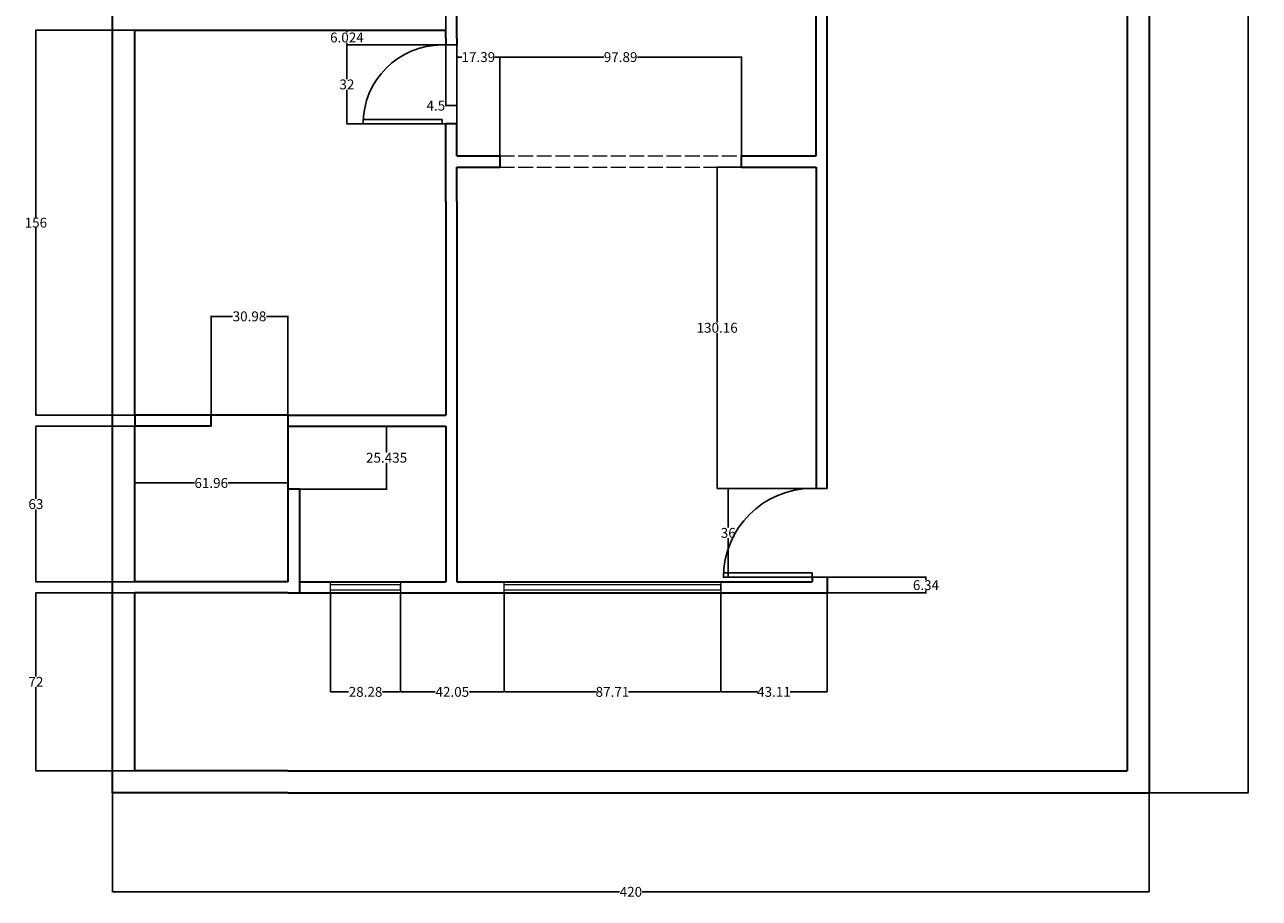
# Model space of a CAD drawing. Units: inches. Extents: x 1353 to 1853, y 16593 to 17433.
# Tile 1 of 4: x 1353 to 1853, y 16593 to 16947. Entities that reach past the tile are written whole.
import ezdxf

# ---------------------------------------------------------------- set-up
doc = ezdxf.new("R2010")
doc.units = ezdxf.units.IN
doc.header["$MEASUREMENT"] = 0
doc.linetypes.add('ACAD_ISO02W100', pattern=[15, 12, -3])
for name, color, linetype, lineweight in [('A-ANNO-DIMS', 2, 'Continuous', 18), ('A-DOOR', 3, 'Continuous', 25), ('A-GLAZ', 4, 'Continuous', 18), ('A-WALL', 7, 'Continuous', 35)]:
    doc.layers.add(name, color=color, linetype=linetype, lineweight=lineweight)
doc.layers.add('A-WALL-OVHD', color=51, linetype='ACAD_ISO02W100', lineweight=18, true_color=0xf8f6b0)
doc.styles.get("Standard").update_dxf_attribs({"font": 'arial.ttf'})
doc.dimstyles.get("Standard").update_dxf_attribs({"dimtxt": 4, "dimasz": 0.18, "dimexe": 0.18, "dimexo": 0.0625, "dimgap": 0.09, "dimtad": 0, "dimtih": 1, "dimtoh": 1, "dimdec": 0, "dimzin": 0, "dimdsep": 46, "dimlunit": 3, "dimtxsty": 'Standard', "dimcen": 0.09, "dimadec": 0, "dimazin": 0, "dimtfac": 1, "dimtdec": 0, "dimtofl": 0, "dimtmove": 0, "dimatfit": 3, "dimfxl": 1, "dimtolj": 1, "dimtzin": 0, "dimarcsym": 0})

# ---------------------------------------------------------------- blocks, each defined once
blk = doc.blocks.new('*U4')
for p, q in [((0, 0), (0, -6)), ((32, 0), (32, -6))]:
    blk.add_line(p, q)
blk.add_lwpolyline([(0, 0), (0, 32), (1.75, 32), (1.75, 0)], close=True)
blk.add_arc((0, 0), 32, 0, 90)
blk = doc.blocks.new('*U3')
for p, q in [((0, 0), (0, -6)), ((36, 0), (36, -6))]:
    blk.add_line(p, q)
blk.add_lwpolyline([(0, 0), (0, 36), (1.75, 36), (1.75, 0)], close=True)
blk.add_arc((0, 0), 36, 0, 90)
blk = doc.blocks.new('*D13')
at = {"layer": 'A-ANNO-DIMS', "color": 0, "lineweight": -2, "transparency": 16777216}
for p, q in [((1388.88, 16635.72), (1388.88, 16595.55)), ((1808.88, 16635.72), (1808.88, 16595.55)), ((1389.06, 16595.73), (1594.3, 16595.73)), ((1808.7, 16595.73), (1603.47, 16595.73))]:
    blk.add_line(p, q, dxfattribs=at)
at = {"layer": 'A-ANNO-DIMS', "color": 0, "transparency": 16777216}
for points in [[(1389.06, 16595.76), (1389.06, 16595.7), (1388.88, 16595.73)], [(1808.7, 16595.76), (1808.7, 16595.7), (1808.88, 16595.73)]]:
    blk.add_solid(points, dxfattribs=at)
at = {"layer": 'Defpoints', "color": 0, "transparency": 16777216}
for p in [(1388.88, 16635.78), (1808.88, 16635.78), (1808.88, 16595.73)]:
    blk.add_point(p, dxfattribs=at)
at = {"layer": 'A-ANNO-DIMS', "color": 0, "transparency": 16777216, "insert": (1598.88, 16595.73), "char_height": 4, "attachment_point": 5}
blk.add_mtext('\\A1;420', dxfattribs=at)
blk = doc.blocks.new('*D14')
at = {"layer": 'A-ANNO-DIMS', "color": 0, "lineweight": -2, "transparency": 16777216}
for p, q in [((1808.95, 17432.78), (1849.11, 17432.78)), ((1848.93, 17432.6), (1848.93, 17036.41)), ((1848.93, 16635.96), (1848.93, 17032.15)), ((1808.95, 16635.78), (1849.11, 16635.78))]:
    blk.add_line(p, q, dxfattribs=at)
at = {"layer": 'A-ANNO-DIMS', "color": 0, "transparency": 16777216}
for points in [[(1848.9, 17432.6), (1848.96, 17432.6), (1848.93, 17432.78)], [(1848.9, 16635.96), (1848.96, 16635.96), (1848.93, 16635.78)]]:
    blk.add_solid(points, dxfattribs=at)
at = {"layer": 'Defpoints', "color": 0, "transparency": 16777216}
for p in [(1808.88, 17432.78), (1848.93, 17432.78), (1808.88, 16635.78)]:
    blk.add_point(p, dxfattribs=at)
at = {"layer": 'A-ANNO-DIMS', "color": 0, "transparency": 16777216, "insert": (1848.93, 17034.28), "char_height": 4, "attachment_point": 5}
blk.add_mtext('\\A1;797', dxfattribs=at)
blk = doc.blocks.new('*D20')
at = {"layer": 'A-ANNO-DIMS', "color": 0, "lineweight": -2, "transparency": 16777216}
for p, q in [((1397.82, 16944.78), (1357.65, 16944.78)), ((1357.83, 16944.6), (1357.83, 16868.91)), ((1357.83, 16788.96), (1357.83, 16864.65)), ((1397.82, 16788.78), (1357.65, 16788.78))]:
    blk.add_line(p, q, dxfattribs=at)
at = {"layer": 'A-ANNO-DIMS', "color": 0, "transparency": 16777216}
for points in [[(1357.8, 16944.6), (1357.86, 16944.6), (1357.83, 16944.78)], [(1357.8, 16788.96), (1357.86, 16788.96), (1357.83, 16788.78)]]:
    blk.add_solid(points, dxfattribs=at)
at = {"layer": 'Defpoints', "color": 0, "transparency": 16777216}
for p in [(1357.83, 16944.78), (1397.88, 16944.78), (1397.88, 16788.78)]:
    blk.add_point(p, dxfattribs=at)
at = {"layer": 'A-ANNO-DIMS', "color": 0, "transparency": 16777216, "insert": (1357.83, 16866.78), "char_height": 4, "attachment_point": 5}
blk.add_mtext('\\A1;156', dxfattribs=at)
blk = doc.blocks.new('*D21')
at = {"layer": 'A-ANNO-DIMS', "color": 0, "lineweight": -2, "transparency": 16777216}
for p, q in [((1397.82, 16784.28), (1357.65, 16784.28)), ((1357.83, 16784.1), (1357.83, 16754.91)), ((1357.83, 16721.46), (1357.83, 16750.65)), ((1397.82, 16721.28), (1357.65, 16721.28))]:
    blk.add_line(p, q, dxfattribs=at)
at = {"layer": 'A-ANNO-DIMS', "color": 0, "transparency": 16777216}
for points in [[(1357.8, 16784.1), (1357.86, 16784.1), (1357.83, 16784.28)], [(1357.8, 16721.46), (1357.86, 16721.46), (1357.83, 16721.28)]]:
    blk.add_solid(points, dxfattribs=at)
at = {"layer": 'Defpoints', "color": 0, "transparency": 16777216}
for p in [(1357.83, 16784.28), (1397.88, 16784.28), (1397.88, 16721.28)]:
    blk.add_point(p, dxfattribs=at)
at = {"layer": 'A-ANNO-DIMS', "color": 0, "transparency": 16777216, "insert": (1357.83, 16752.78), "char_height": 4, "attachment_point": 5}
blk.add_mtext('\\A1;63', dxfattribs=at)
blk = doc.blocks.new('*D22')
at = {"layer": 'A-ANNO-DIMS', "color": 0, "lineweight": -2, "transparency": 16777216}
for p, q in [((1397.82, 16716.78), (1357.65, 16716.78)), ((1357.83, 16716.6), (1357.83, 16682.88)), ((1357.83, 16644.96), (1357.83, 16678.68)), ((1397.82, 16644.78), (1357.65, 16644.78))]:
    blk.add_line(p, q, dxfattribs=at)
at = {"layer": 'A-ANNO-DIMS', "color": 0, "transparency": 16777216}
for points in [[(1357.8, 16716.6), (1357.86, 16716.6), (1357.83, 16716.78)], [(1357.8, 16644.96), (1357.86, 16644.96), (1357.83, 16644.78)]]:
    blk.add_solid(points, dxfattribs=at)
at = {"layer": 'Defpoints', "color": 0, "transparency": 16777216}
for p in [(1357.83, 16716.78), (1397.88, 16716.78), (1397.88, 16644.78)]:
    blk.add_point(p, dxfattribs=at)
at = {"layer": 'A-ANNO-DIMS', "color": 0, "transparency": 16777216, "insert": (1357.83, 16680.78), "char_height": 4, "attachment_point": 5}
blk.add_mtext('\\A1;72', dxfattribs=at)
blk = doc.blocks.new('*D29')
at = {"layer": 'A-ANNO-DIMS', "color": 0, "lineweight": -2, "transparency": 16777216}
for p, q in [((1673.82, 16889.28), (1633.65, 16889.28)), ((1633.83, 16889.1), (1633.83, 16826.33)), ((1633.83, 16759.3), (1633.83, 16822.07)), ((1673.82, 16759.12), (1633.65, 16759.12))]:
    blk.add_line(p, q, dxfattribs=at)
at = {"layer": 'A-ANNO-DIMS', "color": 0, "transparency": 16777216}
for points in [[(1633.8, 16889.1), (1633.86, 16889.1), (1633.83, 16889.28)], [(1633.8, 16759.3), (1633.86, 16759.3), (1633.83, 16759.12)]]:
    blk.add_solid(points, dxfattribs=at)
at = {"layer": 'Defpoints', "color": 0, "transparency": 16777216}
for p in [(1633.83, 16889.28), (1673.88, 16889.28), (1673.88, 16759.12)]:
    blk.add_point(p, dxfattribs=at)
at = {"layer": 'A-ANNO-DIMS', "color": 0, "transparency": 16777216, "insert": (1633.83, 16824.2), "char_height": 4, "attachment_point": 5}
blk.add_mtext('\\A1;130.16', dxfattribs=at)
blk = doc.blocks.new('*D32')
at = {"layer": 'A-ANNO-DIMS', "color": 0, "lineweight": -2, "transparency": 16777216}
for p, q in [((1397.88, 16721.34), (1397.88, 16761.51)), ((1398.06, 16761.33), (1422.02, 16761.33)), ((1459.67, 16761.33), (1435.71, 16761.33)), ((1459.85, 16721.34), (1459.85, 16761.51))]:
    blk.add_line(p, q, dxfattribs=at)
at = {"layer": 'A-ANNO-DIMS', "color": 0, "transparency": 16777216}
for points in [[(1398.06, 16761.36), (1398.06, 16761.3), (1397.88, 16761.33)], [(1459.67, 16761.36), (1459.67, 16761.3), (1459.85, 16761.33)]]:
    blk.add_solid(points, dxfattribs=at)
at = {"layer": 'Defpoints', "color": 0, "transparency": 16777216}
for p in [(1459.85, 16761.33), (1397.88, 16721.28), (1459.85, 16721.28)]:
    blk.add_point(p, dxfattribs=at)
at = {"layer": 'A-ANNO-DIMS', "color": 0, "transparency": 16777216, "insert": (1428.87, 16761.33), "char_height": 4, "attachment_point": 5}
blk.add_mtext('\\A1;61.96', dxfattribs=at)
blk = doc.blocks.new('*D33')
at = {"layer": 'A-ANNO-DIMS', "color": 0, "lineweight": -2, "transparency": 16777216}
for p, q in [((1523.88, 16954.18), (1523.88, 16914.01)), ((1528.38, 16954.18), (1528.38, 16914.01)), ((1523.88, 16914.19), (1523.7, 16914.19)), ((1528.2, 16914.19), (1524.06, 16914.19))]:
    blk.add_line(p, q, dxfattribs=at)
at = {"layer": 'A-ANNO-DIMS', "color": 0, "transparency": 16777216}
for points in [[(1524.06, 16914.22), (1524.06, 16914.16), (1523.88, 16914.19)], [(1528.2, 16914.22), (1528.2, 16914.16), (1528.38, 16914.19)]]:
    blk.add_solid(points, dxfattribs=at)
at = {"layer": 'Defpoints', "color": 0, "transparency": 16777216}
for p in [(1523.88, 16954.24), (1528.38, 16954.24), (1523.88, 16914.19)]:
    blk.add_point(p, dxfattribs=at)
at = {"layer": 'A-ANNO-DIMS', "color": 0, "transparency": 16777216, "insert": (1519.88, 16914.19), "char_height": 4, "attachment_point": 5}
blk.add_mtext('\\A1;4.5', dxfattribs=at)
blk = doc.blocks.new('*D47')
at = {"layer": 'A-ANNO-DIMS', "color": 0, "lineweight": -2, "transparency": 16777216}
for p, q in [((1477.24, 16716.72), (1477.24, 16676.55)), ((1505.52, 16716.72), (1505.52, 16676.55)), ((1477.42, 16676.73), (1484.5, 16676.73)), ((1505.34, 16676.73), (1498.26, 16676.73))]:
    blk.add_line(p, q, dxfattribs=at)
at = {"layer": 'A-ANNO-DIMS', "color": 0, "transparency": 16777216}
for points in [[(1477.42, 16676.76), (1477.42, 16676.7), (1477.24, 16676.73)], [(1505.34, 16676.76), (1505.34, 16676.7), (1505.52, 16676.73)]]:
    blk.add_solid(points, dxfattribs=at)
at = {"layer": 'Defpoints', "color": 0, "transparency": 16777216}
for p in [(1477.24, 16716.78), (1505.52, 16716.78), (1477.24, 16676.73)]:
    blk.add_point(p, dxfattribs=at)
at = {"layer": 'A-ANNO-DIMS', "color": 0, "transparency": 16777216, "insert": (1491.38, 16676.73), "char_height": 4, "attachment_point": 5}
blk.add_mtext('\\A1;28.28', dxfattribs=at)
blk = doc.blocks.new('*D48')
at = {"layer": 'A-ANNO-DIMS', "color": 0, "lineweight": -2, "transparency": 16777216}
for p, q in [((1547.57, 16716.72), (1547.57, 16676.55)), ((1635.28, 16716.72), (1635.28, 16676.55)), ((1547.75, 16676.73), (1584.96, 16676.73)), ((1635.1, 16676.73), (1597.88, 16676.73))]:
    blk.add_line(p, q, dxfattribs=at)
at = {"layer": 'A-ANNO-DIMS', "color": 0, "transparency": 16777216}
for points in [[(1547.75, 16676.76), (1547.75, 16676.7), (1547.57, 16676.73)], [(1635.1, 16676.76), (1635.1, 16676.7), (1635.28, 16676.73)]]:
    blk.add_solid(points, dxfattribs=at)
at = {"layer": 'Defpoints', "color": 0, "transparency": 16777216}
for p in [(1547.57, 16716.78), (1635.28, 16716.78), (1547.57, 16676.73)]:
    blk.add_point(p, dxfattribs=at)
at = {"layer": 'A-ANNO-DIMS', "color": 0, "transparency": 16777216, "insert": (1591.42, 16676.73), "char_height": 4, "attachment_point": 5}
blk.add_mtext('\\A1;87.71', dxfattribs=at)
blk = doc.blocks.new('*D49')
at = {"layer": 'A-ANNO-DIMS', "color": 0, "lineweight": -2, "transparency": 16777216}
for p, q in [((1505.52, 16716.72), (1505.52, 16676.55)), ((1547.57, 16716.72), (1547.57, 16676.55)), ((1505.7, 16676.73), (1519.61, 16676.73)), ((1547.39, 16676.73), (1533.48, 16676.73))]:
    blk.add_line(p, q, dxfattribs=at)
at = {"layer": 'A-ANNO-DIMS', "color": 0, "transparency": 16777216}
for points in [[(1505.7, 16676.76), (1505.7, 16676.7), (1505.52, 16676.73)], [(1547.39, 16676.76), (1547.39, 16676.7), (1547.57, 16676.73)]]:
    blk.add_solid(points, dxfattribs=at)
at = {"layer": 'Defpoints', "color": 0, "transparency": 16777216}
for p in [(1505.52, 16716.78), (1547.57, 16716.78), (1505.52, 16676.73)]:
    blk.add_point(p, dxfattribs=at)
at = {"layer": 'A-ANNO-DIMS', "color": 0, "transparency": 16777216, "insert": (1526.54, 16676.73), "char_height": 4, "attachment_point": 5}
blk.add_mtext('\\A1;42.05', dxfattribs=at)
blk = doc.blocks.new('*D50')
at = {"layer": 'A-ANNO-DIMS', "color": 0, "lineweight": -2, "transparency": 16777216}
for p, q in [((1635.28, 16716.72), (1635.28, 16676.55)), ((1678.38, 16716.72), (1678.38, 16676.55)), ((1635.46, 16676.73), (1650.3, 16676.73)), ((1678.2, 16676.73), (1663.36, 16676.73))]:
    blk.add_line(p, q, dxfattribs=at)
at = {"layer": 'A-ANNO-DIMS', "color": 0, "transparency": 16777216}
for points in [[(1635.46, 16676.76), (1635.46, 16676.7), (1635.28, 16676.73)], [(1678.2, 16676.76), (1678.2, 16676.7), (1678.38, 16676.73)]]:
    blk.add_solid(points, dxfattribs=at)
at = {"layer": 'Defpoints', "color": 0, "transparency": 16777216}
for p in [(1635.28, 16716.78), (1678.38, 16716.78), (1635.28, 16676.73)]:
    blk.add_point(p, dxfattribs=at)
at = {"layer": 'A-ANNO-DIMS', "color": 0, "transparency": 16777216, "insert": (1656.83, 16676.73), "char_height": 4, "attachment_point": 5}
blk.add_mtext('\\A1;43.11', dxfattribs=at)
blk = doc.blocks.new('*D60')
at = {"layer": 'A-ANNO-DIMS', "color": 0, "lineweight": -2, "transparency": 16777216}
for p, q in [((1523.82, 16938.76), (1483.65, 16938.76)), ((1483.83, 16938.58), (1483.83, 16924.89)), ((1483.83, 16906.94), (1483.83, 16920.62)), ((1523.82, 16906.76), (1483.65, 16906.76))]:
    blk.add_line(p, q, dxfattribs=at)
at = {"layer": 'A-ANNO-DIMS', "color": 0, "transparency": 16777216}
for points in [[(1483.8, 16938.58), (1483.86, 16938.58), (1483.83, 16938.76)], [(1483.8, 16906.94), (1483.86, 16906.94), (1483.83, 16906.76)]]:
    blk.add_solid(points, dxfattribs=at)
at = {"layer": 'Defpoints', "color": 0, "transparency": 16777216}
for p in [(1483.83, 16938.76), (1523.88, 16938.76), (1523.88, 16906.76)]:
    blk.add_point(p, dxfattribs=at)
at = {"layer": 'A-ANNO-DIMS', "color": 0, "transparency": 16777216, "insert": (1483.83, 16922.76), "char_height": 4, "attachment_point": 5}
blk.add_mtext('\\A1;32', dxfattribs=at)
blk = doc.blocks.new('*D63')
at = {"layer": 'A-ANNO-DIMS', "color": 0, "lineweight": -2, "transparency": 16777216}
for p, q in [((1678.32, 16759.12), (1638.15, 16759.12)), ((1638.33, 16758.94), (1638.33, 16743.25)), ((1638.33, 16723.3), (1638.33, 16738.99)), ((1678.32, 16723.12), (1638.15, 16723.12))]:
    blk.add_line(p, q, dxfattribs=at)
at = {"layer": 'A-ANNO-DIMS', "color": 0, "transparency": 16777216}
for points in [[(1638.3, 16758.94), (1638.36, 16758.94), (1638.33, 16759.12)], [(1638.3, 16723.3), (1638.36, 16723.3), (1638.33, 16723.12)]]:
    blk.add_solid(points, dxfattribs=at)
at = {"layer": 'Defpoints', "color": 0, "transparency": 16777216}
for p in [(1638.33, 16759.12), (1678.38, 16759.12), (1678.38, 16723.12)]:
    blk.add_point(p, dxfattribs=at)
at = {"layer": 'A-ANNO-DIMS', "color": 0, "transparency": 16777216, "insert": (1638.33, 16741.12), "char_height": 4, "attachment_point": 5}
blk.add_mtext('\\A1;36', dxfattribs=at)
blk = doc.blocks.new('*D64')
at = {"layer": 'A-ANNO-DIMS', "color": 0, "lineweight": -2, "transparency": 16777216}
for p, q in [((1545.78, 16893.84), (1545.78, 16934.01)), ((1545.96, 16933.83), (1587.88, 16933.83)), ((1643.48, 16933.83), (1601.56, 16933.83)), ((1643.66, 16893.84), (1643.66, 16934.01))]:
    blk.add_line(p, q, dxfattribs=at)
at = {"layer": 'A-ANNO-DIMS', "color": 0, "transparency": 16777216}
for points in [[(1545.96, 16933.86), (1545.96, 16933.8), (1545.78, 16933.83)], [(1643.48, 16933.86), (1643.48, 16933.8), (1643.66, 16933.83)]]:
    blk.add_solid(points, dxfattribs=at)
at = {"layer": 'Defpoints', "color": 0, "transparency": 16777216}
for p in [(1643.66, 16933.83), (1545.78, 16893.78), (1643.66, 16893.78)]:
    blk.add_point(p, dxfattribs=at)
at = {"layer": 'A-ANNO-DIMS', "color": 0, "transparency": 16777216, "insert": (1594.72, 16933.83), "char_height": 4, "attachment_point": 5}
blk.add_mtext('\\A1;97.89', dxfattribs=at)
blk = doc.blocks.new('*D65')
at = {"layer": 'A-ANNO-DIMS', "color": 0, "lineweight": -2, "transparency": 16777216}
for p, q in [((1528.38, 16893.84), (1528.38, 16934.01)), ((1528.56, 16933.83), (1530.43, 16933.83)), ((1545.6, 16933.83), (1543.73, 16933.83)), ((1545.78, 16893.84), (1545.78, 16934.01))]:
    blk.add_line(p, q, dxfattribs=at)
at = {"layer": 'A-ANNO-DIMS', "color": 0, "transparency": 16777216}
for points in [[(1528.56, 16933.86), (1528.56, 16933.8), (1528.38, 16933.83)], [(1545.6, 16933.86), (1545.6, 16933.8), (1545.78, 16933.83)]]:
    blk.add_solid(points, dxfattribs=at)
at = {"layer": 'Defpoints', "color": 0, "transparency": 16777216}
for p in [(1545.78, 16933.83), (1528.38, 16893.78), (1545.78, 16893.78)]:
    blk.add_point(p, dxfattribs=at)
at = {"layer": 'A-ANNO-DIMS', "color": 0, "transparency": 16777216, "insert": (1537.08, 16933.83), "char_height": 4, "attachment_point": 5}
blk.add_mtext('\\A1;17.39', dxfattribs=at)
blk = doc.blocks.new('*D66')
at = {"layer": 'A-ANNO-DIMS', "color": 0, "lineweight": -2, "transparency": 16777216}
for p, q in [((1428.87, 16788.84), (1428.87, 16829.01)), ((1429.05, 16828.83), (1437.51, 16828.83)), ((1459.67, 16828.83), (1451.2, 16828.83)), ((1459.85, 16788.84), (1459.85, 16829.01))]:
    blk.add_line(p, q, dxfattribs=at)
at = {"layer": 'A-ANNO-DIMS', "color": 0, "transparency": 16777216}
for points in [[(1429.05, 16828.86), (1429.05, 16828.8), (1428.87, 16828.83)], [(1459.67, 16828.86), (1459.67, 16828.8), (1459.85, 16828.83)]]:
    blk.add_solid(points, dxfattribs=at)
at = {"layer": 'Defpoints', "color": 0, "transparency": 16777216}
for p in [(1459.85, 16828.83), (1428.87, 16788.78), (1459.85, 16788.78)]:
    blk.add_point(p, dxfattribs=at)
at = {"layer": 'A-ANNO-DIMS', "color": 0, "transparency": 16777216, "insert": (1444.36, 16828.83), "char_height": 4, "attachment_point": 5}
blk.add_mtext('\\A1;30.98', dxfattribs=at)
blk = doc.blocks.new('*D67')
at = {"layer": 'A-ANNO-DIMS', "color": 0, "lineweight": -2, "transparency": 16777216}
for p, q in [((1459.91, 16784.28), (1500.08, 16784.28)), ((1499.9, 16784.1), (1499.9, 16773.7)), ((1499.9, 16759.03), (1499.9, 16769.43)), ((1459.91, 16758.85), (1500.08, 16758.85))]:
    blk.add_line(p, q, dxfattribs=at)
at = {"layer": 'A-ANNO-DIMS', "color": 0, "transparency": 16777216}
for points in [[(1499.87, 16784.1), (1499.93, 16784.1), (1499.9, 16784.28)], [(1499.87, 16759.03), (1499.93, 16759.03), (1499.9, 16758.85)]]:
    blk.add_solid(points, dxfattribs=at)
at = {"layer": 'Defpoints', "color": 0, "transparency": 16777216}
for p in [(1459.85, 16784.28), (1459.85, 16758.85), (1499.9, 16758.85)]:
    blk.add_point(p, dxfattribs=at)
at = {"layer": 'A-ANNO-DIMS', "color": 0, "transparency": 16777216, "insert": (1499.9, 16771.56), "char_height": 4, "attachment_point": 5}
blk.add_mtext('\\A1;25.435', dxfattribs=at)
blk = doc.blocks.new('*D77')
at = {"layer": 'A-ANNO-DIMS', "color": 0, "lineweight": -2, "transparency": 16777216}
for p, q in [((1523.82, 16944.78), (1483.65, 16944.78)), ((1483.83, 16944.6), (1483.83, 16943.9)), ((1523.82, 16938.76), (1483.65, 16938.76)), ((1483.83, 16938.94), (1483.83, 16939.64))]:
    blk.add_line(p, q, dxfattribs=at)
at = {"layer": 'A-ANNO-DIMS', "color": 0, "transparency": 16777216}
for points in [[(1483.8, 16944.6), (1483.86, 16944.6), (1483.83, 16944.78)], [(1483.8, 16938.94), (1483.86, 16938.94), (1483.83, 16938.76)]]:
    blk.add_solid(points, dxfattribs=at)
at = {"layer": 'Defpoints', "color": 0, "transparency": 16777216}
for p in [(1483.83, 16944.78), (1523.88, 16944.78), (1523.88, 16938.76)]:
    blk.add_point(p, dxfattribs=at)
at = {"layer": 'A-ANNO-DIMS', "color": 0, "transparency": 16777216, "insert": (1483.83, 16941.77), "char_height": 4, "attachment_point": 5}
blk.add_mtext('\\A1;6.024', dxfattribs=at)
blk = doc.blocks.new('*D79')
at = {"layer": 'A-ANNO-DIMS', "color": 0, "lineweight": -2, "transparency": 16777216}
for p, q in [((1678.45, 16723.12), (1718.61, 16723.12)), ((1718.43, 16722.94), (1718.43, 16722.08)), ((1678.45, 16716.78), (1718.61, 16716.78)), ((1718.43, 16716.96), (1718.43, 16717.82))]:
    blk.add_line(p, q, dxfattribs=at)
at = {"layer": 'A-ANNO-DIMS', "color": 0, "transparency": 16777216}
for points in [[(1718.4, 16722.94), (1718.46, 16722.94), (1718.43, 16723.12)], [(1718.4, 16716.96), (1718.46, 16716.96), (1718.43, 16716.78)]]:
    blk.add_solid(points, dxfattribs=at)
at = {"layer": 'Defpoints', "color": 0, "transparency": 16777216}
for p in [(1678.38, 16723.12), (1678.38, 16716.78), (1718.43, 16716.78)]:
    blk.add_point(p, dxfattribs=at)
at = {"layer": 'A-ANNO-DIMS', "color": 0, "transparency": 16777216, "insert": (1718.43, 16719.95), "char_height": 4, "attachment_point": 5}
blk.add_mtext('\\A1;6.34', dxfattribs=at)

msp = doc.modelspace()

# ---------------------------------------------------------------- linework, layer by layer
at = {"layer": 'A-GLAZ'}
for p, q in [((1477.2369, 16716.7809), (1477.2369, 16721.2809)), ((1477.2369, 16721.2809), (1505.5194, 16721.2809)), ((1505.5194, 16721.2809), (1505.5194, 16716.7809)), ((1547.5656, 16716.7809), (1547.5656, 16721.2809)), ((1547.5656, 16721.2809), (1635.2751, 16721.2809)), ((1635.2751, 16721.2809), (1635.2751, 16721.2809)), ((1635.2751, 16721.2809), (1635.2751, 16716.7809)), ((1505.5194, 16720.0396), (1477.2369, 16720.0396)), ((1477.2369, 16720.0396), (1477.2369, 16720.0396)), ((1477.2369, 16716.7809), (1477.2369, 16718.023)), ((1477.2369, 16718.023), (1505.5194, 16718.023)), ((1505.5194, 16716.7809), (1477.2369, 16716.7809)), ((1505.5194, 16718.023), (1505.5194, 16720.0396)), ((1635.2751, 16720.0306), (1547.5656, 16720.0306)), ((1547.5656, 16716.7809), (1547.5656, 16718.014)), ((1547.5656, 16718.014), (1635.2751, 16718.014)), ((1635.2751, 16716.7809), (1547.5656, 16716.7809)), ((1635.2751, 16718.014), (1635.2751, 16720.0306))]:
    msp.add_line(p, q, dxfattribs=at)
at = {"layer": 'A-WALL'}
for p, q in [((1388.8844, 16635.7809), (1388.8844, 17432.7809)), ((1808.8844, 17432.7809), (1808.8844, 16635.7809)), ((1799.8844, 17087.7809), (1799.8844, 16644.7809)), ((1673.8844, 16893.7809), (1673.8844, 17047.277)), ((1678.3844, 16759.1207), (1678.3844, 17047.277)), ((1528.3844, 16944.7809), (1528.3844, 16954.2398)), ((1397.8844, 16944.7809), (1459.8459, 16944.7809)), ((1397.8844, 16875.2834), (1397.8844, 16944.7809)), ((1459.8459, 16944.7809), (1523.8844, 16944.7809)), ((1523.8844, 16941.5554), (1523.8844, 16944.7809)), ((1523.8844, 16941.5554), (1523.8844, 16938.7569)), ((1528.3844, 16941.5554), (1528.3844, 16944.7809)), ((1528.3844, 16941.5554), (1528.3844, 16938.7569)), ((1523.8844, 16875.2834), (1523.8844, 16906.7569)), ((1528.3844, 16906.7569), (1523.8844, 16906.7569)), ((1528.3844, 16893.7809), (1528.3844, 16906.7569)), ((1528.3844, 16893.7809), (1545.7758, 16893.7809)), ((1545.7758, 16893.7809), (1545.7758, 16889.2809)), ((1643.664, 16889.2809), (1643.664, 16893.7809)), ((1643.664, 16893.7809), (1673.8844, 16893.7809)), ((1528.3844, 16875.2834), (1528.3844, 16889.2809)), ((1528.3844, 16889.2809), (1545.7758, 16889.2809)), ((1643.664, 16889.2809), (1673.8844, 16889.2809)), ((1673.8844, 16889.2809), (1673.8844, 16763.1207)), ((1397.8844, 16788.7809), (1397.8844, 16877.2809)), ((1523.8844, 16875.2834), (1523.8844, 16788.7809)), ((1528.3844, 16875.2834), (1528.3844, 16784.2809)), ((1459.8459, 16788.7809), (1397.8844, 16788.7809)), ((1428.8651, 16788.7809), (1397.8844, 16788.7809)), ((1397.8844, 16788.7809), (1397.8844, 16784.2809)), ((1428.8651, 16784.2809), (1428.8651, 16788.7809)), ((1459.8459, 16788.7809), (1523.8844, 16788.7809)), ((1459.8459, 16788.7809), (1459.8459, 16721.2809)), ((1428.8651, 16784.2809), (1397.8844, 16784.2809)), ((1397.8844, 16721.2809), (1397.8844, 16784.2809)), ((1459.8459, 16784.2809), (1523.8844, 16784.2809)), ((1523.8844, 16784.2809), (1523.8844, 16721.2809)), ((1528.3844, 16784.2809), (1528.3844, 16721.2809)), ((1673.8844, 16763.1207), (1673.8844, 16759.1207)), ((1464.8177, 16758.8459), (1459.8459, 16758.8459)), ((1464.8177, 16716.7809), (1464.8177, 16758.8459)), ((1459.8459, 16721.2809), (1397.8844, 16721.2809)), ((1464.8177, 16721.2809), (1523.8844, 16721.2809)), ((1528.3844, 16721.2809), (1672.3844, 16721.2809)), ((1672.3844, 16721.2809), (1672.1111, 16721.2809)), ((1672.3844, 16723.1207), (1672.3844, 16721.2809)), ((1678.3844, 16723.1207), (1678.3844, 16716.7809)), ((1397.8844, 16644.7809), (1397.8844, 16716.7809)), ((1459.8459, 16716.7809), (1397.8844, 16716.7809)), ((1459.8459, 16716.7809), (1678.3844, 16716.7809)), ((1459.8459, 16716.7809), (1464.8177, 16716.7809)), ((1459.8459, 16644.7809), (1397.8844, 16644.7809)), ((1459.8459, 16644.7809), (1528.3844, 16644.7809)), ((1528.3844, 16644.7809), (1678.3844, 16644.7809)), ((1678.3844, 16644.7809), (1799.8844, 16644.7809)), ((1397.8844, 16635.7809), (1388.8844, 16635.7809)), ((1459.8459, 16635.7809), (1397.8844, 16635.7809)), ((1459.8459, 16635.7809), (1528.3844, 16635.7809)), ((1528.3844, 16635.7809), (1808.8844, 16635.7809))]:
    msp.add_line(p, q, dxfattribs=at)
at = {"layer": 'A-WALL-OVHD', "ltscale": 0.5}
for p, q in [((1545.7758, 16893.7809), (1643.664, 16893.7809)), ((1545.7758, 16889.2809), (1643.664, 16889.2809))]:
    msp.add_line(p, q, dxfattribs=at)

# ---------------------------------------------------------------- block references
at = {"layer": 'A-DOOR', "rotation": 90}
for name, p in [('*U4', (1522.3844, 16906.7569)), ('*U3', (1672.3844, 16723.1207))]:
    msp.add_blockref(name, p, dxfattribs=at)

# ---------------------------------------------------------------- dimensions: what is measured, and where the dimension line sits
at = {"layer": 'A-ANNO-DIMS'}
for base, p1, p2, angle, override, picture, middle in [((1848.9344, 17432.7809), (1808.8844, 16635.7809), (1808.8844, 17432.7809), 90, {"dimdec": 0, "dimlfac": 1, "dimrnd": 0, "dimzin": 0, "dimdsep": 46, "dimlunit": 2}, '*D14', (1848.9344, 17034.2809)), ((1523.8844, 16914.1898), (1528.3844, 16954.2398), (1523.8844, 16954.2398), 180, {"dimdec": 1, "dimlfac": 1, "dimrnd": 0, "dimzin": 0, "dimdsep": 46, "dimlunit": 2}, '*D33', (1519.8777, 16914.1898)), ((1357.8344, 16944.7809), (1397.8844, 16788.7809), (1397.8844, 16944.7809), 90, {"dimdec": 0, "dimlfac": 1, "dimrnd": 0, "dimzin": 0, "dimdsep": 46, "dimlunit": 2}, '*D20', (1357.8344, 16866.7809)), ((1483.8344, 16944.7809), (1523.8844, 16938.7569), (1523.8844, 16944.7809), 90, {"dimdec": 3, "dimlfac": 1, "dimrnd": 0, "dimzin": 0, "dimdsep": 46, "dimlunit": 2}, '*D77', (1483.8344, 16941.7689)), ((1483.8344, 16938.7569), (1523.8844, 16906.7569), (1523.8844, 16938.7569), 90, {"dimdec": 0, "dimlfac": 1, "dimrnd": 0, "dimzin": 0, "dimdsep": 46, "dimlunit": 2}, '*D60', (1483.8344, 16922.7569)), ((1633.8344, 16889.2809), (1673.8844, 16759.1207), (1673.8844, 16889.2809), 90, {"dimdec": 2, "dimlfac": 1, "dimrnd": 0, "dimzin": 0, "dimdsep": 46, "dimlunit": 2}, '*D29', (1633.8344, 16824.2008)), ((1357.8344, 16784.2809), (1397.8844, 16721.2809), (1397.8844, 16784.2809), 90, {"dimdec": 0, "dimlfac": 1, "dimrnd": 0, "dimzin": 0, "dimdsep": 46, "dimlunit": 2}, '*D21', (1357.8344, 16752.7809)), ((1499.8959, 16758.8459), (1459.8459, 16784.2809), (1459.8459, 16758.8459), 270, {"dimdec": 3, "dimlfac": 1, "dimrnd": 0, "dimzin": 0, "dimdsep": 46, "dimlunit": 2}, '*D67', (1499.8959, 16771.5634)), ((1638.3344, 16759.1207), (1678.3844, 16723.1207), (1678.3844, 16759.1207), 90, {"dimdec": 0, "dimlfac": 1, "dimrnd": 0, "dimzin": 0, "dimdsep": 46, "dimlunit": 2}, '*D63', (1638.3344, 16741.1207)), ((1718.4344, 16716.7809), (1678.3844, 16723.1207), (1678.3844, 16716.7809), 270, {"dimdec": 2, "dimlfac": 1, "dimrnd": 0, "dimzin": 0, "dimdsep": 46, "dimlunit": 2}, '*D79', (1718.4344, 16719.9508)), ((1357.8344, 16716.7809), (1397.8844, 16644.7809), (1397.8844, 16716.7809), 90, {"dimdec": 0, "dimlfac": 1, "dimrnd": 0, "dimzin": 0, "dimdsep": 46, "dimlunit": 2}, '*D22', (1357.8344, 16680.7809)), ((1477.2369, 16676.7309), (1505.5194, 16716.7809), (1477.2369, 16716.7809), 180, {"dimdec": 2, "dimlfac": 1, "dimrnd": 0, "dimzin": 0, "dimdsep": 46, "dimlunit": 2}, '*D47', (1491.3781, 16676.7309)), ((1505.5194, 16676.7309), (1547.5656, 16716.7809), (1505.5194, 16716.7809), 180, {"dimdec": 2, "dimlfac": 1, "dimrnd": 0, "dimzin": 0, "dimdsep": 46, "dimlunit": 2}, '*D49', (1526.5425, 16676.7309)), ((1547.5656, 16676.7309), (1635.2751, 16716.7809), (1547.5656, 16716.7809), 180, {"dimdec": 2, "dimlfac": 1, "dimrnd": 0, "dimzin": 0, "dimdsep": 46, "dimlunit": 2}, '*D48', (1591.4204, 16676.7309)), ((1635.2751, 16676.7309), (1678.3844, 16716.7809), (1635.2751, 16716.7809), 180, {"dimdec": 2, "dimlfac": 1, "dimrnd": 0, "dimzin": 0, "dimdsep": 46, "dimlunit": 2}, '*D50', (1656.8298, 16676.7309))]:
    dim = msp.add_linear_dim(base=base, p1=p1, p2=p2, angle=angle, dimstyle='Standard', override=override, dxfattribs=at)
    dim.commit()
    dim.dimension.update_dxf_attribs({"geometry": picture, "text_midpoint": middle})
for base, p1, p2, override, picture, middle in [((1545.7758, 16933.8309), (1528.3844, 16893.7809), (1545.7758, 16893.7809), {"dimdec": 2, "dimlfac": 1, "dimrnd": 0, "dimzin": 0, "dimdsep": 46, "dimlunit": 2}, '*D65', (1537.0801, 16933.8309)), ((1643.664, 16933.8309), (1545.7758, 16893.7809), (1643.664, 16893.7809), {"dimdec": 2, "dimlfac": 1, "dimrnd": 0, "dimzin": 0, "dimdsep": 46, "dimlunit": 2}, '*D64', (1594.7199, 16933.8309)), ((1459.8459, 16828.8309), (1428.8651, 16788.7809), (1459.8459, 16788.7809), {"dimdec": 2, "dimlfac": 1, "dimrnd": 0, "dimzin": 0, "dimdsep": 46, "dimlunit": 2}, '*D66', (1444.3555, 16828.8309)), ((1459.8459, 16761.3309), (1397.8844, 16721.2809), (1459.8459, 16721.2809), {"dimdec": 2, "dimlfac": 1, "dimrnd": 0, "dimzin": 0, "dimdsep": 46, "dimlunit": 2}, '*D32', (1428.8651, 16761.3309)), ((1808.8844, 16595.7309), (1388.8844, 16635.7809), (1808.8844, 16635.7809), {"dimdec": 0, "dimlfac": 1, "dimrnd": 0, "dimzin": 0, "dimdsep": 46, "dimlunit": 2}, '*D13', (1598.8844, 16595.7309))]:
    dim = msp.add_linear_dim(base=base, p1=p1, p2=p2, dimstyle='Standard', override=override, dxfattribs=at)
    dim.commit()
    dim.dimension.update_dxf_attribs({"geometry": picture, "text_midpoint": middle})

doc.saveas('drawing.dxf')
